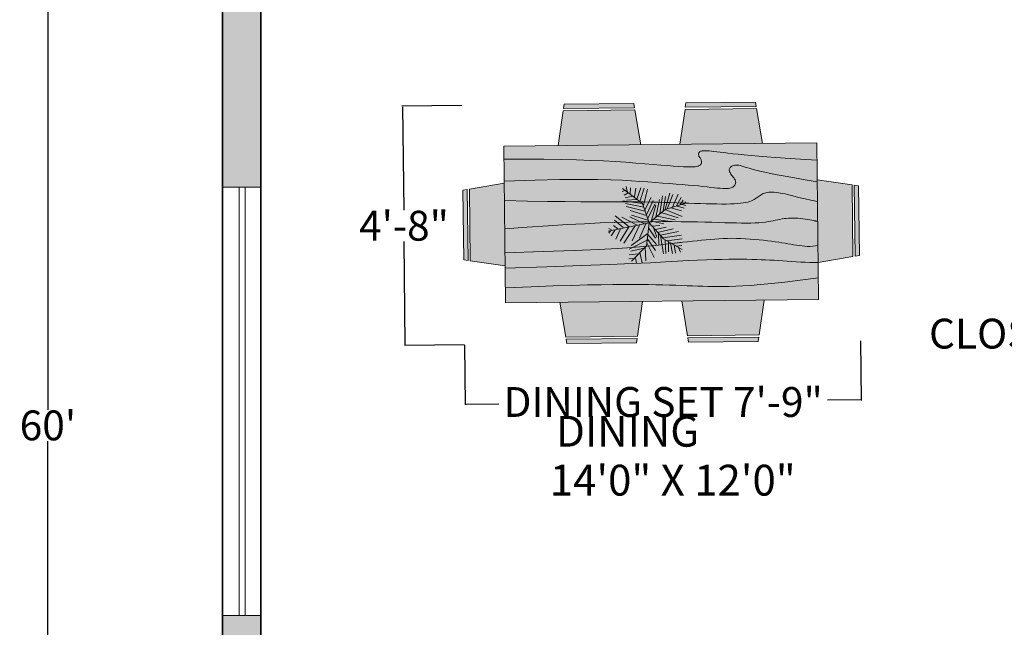
# Model space of a CAD drawing. Units: inches. Extents: x 2167 to 2589, y 1680 to 2489.
# Tile 32 of 38: x 2167 to 2399, y 2000 to 2143. Entities that reach past the tile are written whole.
import ezdxf

# ---------------------------------------------------------------- set-up
doc = ezdxf.new("R2010")
doc.units = ezdxf.units.IN
doc.header["$MEASUREMENT"] = 0
doc.layers.get('0').update_dxf_attribs({"color": 250})
for name, color, linetype, lineweight in [('A-ANNO-DIMS', 2, 'Continuous', 18), ('A-AREA-IDEN', 7, 'Continuous', 18), ('A-FURN-PATT', 31, 'Continuous', 13), ('A-WALL-PATT', 250, 'Continuous', 13), ('C-PROP', 7, 'Continuous', 35), ('furniture', 34, 'Continuous', 18), ('L-PLNT', 106, 'Continuous', 13), ('walls', 7, 'Continuous', 35), ('windows', 141, 'Continuous', 18)]:
    doc.layers.add(name, color=color, linetype=linetype, lineweight=lineweight)
doc.styles.get("Standard").update_dxf_attribs({"font": 'arial.ttf'})
doc.dimstyles.get("Standard").update_dxf_attribs({"dimtxt": 7, "dimasz": 0.18, "dimexe": 0.18, "dimexo": 0.0625, "dimgap": 0.09, "dimtad": 0, "dimtih": 1, "dimtoh": 1, "dimdec": 1, "dimzin": 0, "dimdsep": 46, "dimlunit": 3, "dimtxsty": 'Standard', "dimcen": 0.09, "dimadec": 0, "dimazin": 0, "dimtfac": 1, "dimtdec": 1, "dimtofl": 0, "dimtmove": 0, "dimatfit": 3, "dimfxl": 1, "dimtolj": 1, "dimtzin": 0, "dimarcsym": 0})

# ---------------------------------------------------------------- blocks, each defined once
blk = doc.blocks.new('Dining Set - 36 x 72 in.')
for p, q in [((-22, 27.5), (-22.1562, 26.50042)), ((-22, 27.5), (-6, 27.5)), ((-5.8437, 26.49966), (-6, 27.5)), ((6, 27.5), (5.8438, 26.50042)), ((6, 27.5), (22, 27.5)), ((22.1563, 26.49966), (22, 27.5)), ((-22.2343, 26.00059), (-23.4847, 17.99762)), ((-22.2304, 26), (-5.7608, 26)), ((-5.8416, 26.5), (-22.1534, 26.5)), ((-4.5152, 17.99762), (-5.7655, 25.99926)), ((5.7657, 26.00059), (4.5153, 17.99762)), ((5.7696, 26), (22.2392, 26)), ((22.1584, 26.5), (5.8466, 26.5)), ((23.4848, 17.99762), (22.2345, 25.99926)), ((36, 18), (-36, 18)), ((-36, 18), (-36, -18)), ((36, -18), (36, 18)), ((-44.0006, 8.23428), (-35.9976, 9.48474)), ((44.0006, 8.23428), (35.9976, 9.48474)), ((-45.5, 8), (-44.5004, 8.15617)), ((-45.5, 8), (-45.5, -8)), ((-44.5, -8.15843), (-44.5, 8.15338)), ((-44, 8.23041), (-44, -8.23915)), ((44, 8.23041), (44, -8.23915)), ((44.5, -8.15843), (44.5, 8.15338)), ((45.5, 8), (44.5005, 8.15617)), ((45.5, 8), (45.5, -8)), ((-44.4997, -8.15631), (-45.5, -8)), ((-35.9976, -9.48476), (-43.9993, -8.2345)), ((35.9976, -9.48476), (43.9993, -8.2345)), ((44.4997, -8.15631), (45.5, -8)), ((-36, -18), (36, -18)), ((-22.2343, -26.0006), (-23.4847, -17.99762)), ((-4.5152, -17.99762), (-5.7655, -25.99928)), ((5.7657, -26.0006), (4.5153, -17.99762)), ((23.4848, -17.99762), (22.2345, -25.99928)), ((-22.2304, -26), (-5.7608, -26)), ((-22, -27.5), (-22.1562, -26.50044)), ((-5.8416, -26.5), (-22.1534, -26.5)), ((-5.8437, -26.49967), (-6, -27.5)), ((5.7696, -26), (22.2392, -26)), ((6, -27.5), (5.8438, -26.50044)), ((22.1584, -26.5), (5.8466, -26.5)), ((22.1563, -26.49967), (22, -27.5)), ((-22, -27.5), (-6, -27.5)), ((6, -27.5), (22, -27.5))]:
    blk.add_line(p, q)
for points in [[(-36, 15), (-31.1772, 14.97754), (-26.8079, 14.91406), (-22.8538, 14.81543), (-19.276, 14.6875), (-16.0362, 14.53613), (-13.0957, 14.36718), (-10.4159, 14.18652), (-7.9583, 14), (-5.6904, 13.81315), (-3.6035, 13.63021), (-1.6954, 13.45508), (0.0365, 13.29166), (1.5945, 13.14388), (2.9811, 13.01562), (4.1988, 12.9108), (5.25, 12.83333), (6.1393, 12.78613), (6.8802, 12.76823), (7.4883, 12.77767), (7.9792, 12.8125), (8.3685, 12.87077), (8.6719, 12.95052), (8.9049, 13.0498), (9.0833, 13.16666), (9.2205, 13.29899), (9.3216, 13.44401), (9.3895, 13.59879), (9.4271, 13.76041), (9.4373, 13.92594), (9.4232, 14.09245), (9.3875, 14.257), (9.3333, 14.41666), (9.2638, 14.56917), (9.1836, 14.71484), (9.0975, 14.85465), (9.0104, 14.98958), (8.9272, 15.1206), (8.8529, 15.2487), (8.7922, 15.37483), (8.75, 15.5), (8.7305, 15.62467), (8.7344, 15.74739), (8.7617, 15.86621), (8.8125, 15.97916), (8.8867, 16.08431), (8.9844, 16.17968), (9.1055, 16.26334), (9.25, 16.33333), (9.4189, 16.38802), (9.6172, 16.42708), (9.8506, 16.45052), (10.125, 16.45833), (10.4463, 16.45052), (10.8203, 16.42708), (11.2529, 16.38802), (11.75, 16.33333), (12.3184, 16.26318), (12.9694, 16.17838), (13.7151, 16.07991), (14.5677, 15.96875), (15.5395, 15.84586), (16.6426, 15.71224), (17.8893, 15.56884), (19.2917, 15.41666), (20.859, 15.25667), (22.5879, 15.08984), (24.4721, 14.91715), (26.5052, 14.73958), (28.6809, 14.5581), (30.9929, 14.3737), (33.4347, 14.18733), (36, 14)], [(-36, 10), (-28.9766, 10.14274), (-23.1725, 10.20442), (-18.4241, 10.19775), (-14.5677, 10.13541), (-11.4399, 10.03011), (-8.877, 9.89453), (-6.7154, 9.74137), (-4.7917, 9.58333), (-2.9698, 9.43082), (-1.2246, 9.28515), (0.4415, 9.14534), (2.026, 9.01041), (3.5266, 8.87939), (4.9408, 8.7513), (6.266, 8.62516), (7.5, 8.5), (8.6411, 8.37549), (9.6914, 8.2539), (10.6538, 8.13818), (11.5312, 8.03125), (12.3267, 7.93603), (13.043, 7.85547), (13.6831, 7.79248), (14.25, 7.75), (14.7471, 7.7303), (15.1797, 7.73307), (15.5537, 7.75732), (15.875, 7.80208), (16.1494, 7.86637), (16.3828, 7.94922), (16.5811, 8.04964), (16.75, 8.16666), (16.8944, 8.29915), (17.0143, 8.44531), (17.1089, 8.60319), (17.1771, 8.77083), (17.218, 8.94629), (17.2305, 9.1276), (17.2137, 9.31282), (17.1667, 9.5), (17.0895, 9.6875), (16.987, 9.875), (16.8649, 10.0625), (16.7292, 10.25), (16.5856, 10.4375), (16.4401, 10.625), (16.2985, 10.8125), (16.1667, 11), (16.05, 11.18733), (15.9518, 11.3737), (15.8752, 11.5581), (15.8229, 11.73958), (15.798, 11.91715), (15.8034, 12.08984), (15.842, 12.25667), (15.9167, 12.41666), (16.0295, 12.56836), (16.1784, 12.70833), (16.3605, 12.83268), (16.5729, 12.9375), (16.8127, 13.01888), (17.0768, 13.07291), (17.3625, 13.0957), (17.6667, 13.08333), (17.9894, 13.03312), (18.3418, 12.94726), (18.7382, 12.82918), (19.1927, 12.68229), (19.7195, 12.51001), (20.3327, 12.31575), (21.0465, 12.10294), (21.875, 11.875), (22.8357, 11.63354), (23.959, 11.37304), (25.2786, 11.08618), (26.8282, 10.76562), (28.6414, 10.40405), (30.752, 9.99414), (33.1936, 9.52856), (36, 9)], [(-36, 5.5), (-30.7157, 5.3348), (-26.069, 5.20963), (-21.9946, 5.11767), (-18.4271, 5.05208), (-15.3009, 5.00602), (-12.5508, 4.97265), (-10.1112, 4.94515), (-7.9167, 4.91666), (-5.909, 4.88167), (-4.0586, 4.83984), (-2.3429, 4.79215), (-0.7396, 4.73958), (0.7739, 4.6831), (2.22, 4.6237), (3.6213, 4.56233), (5, 4.5), (6.373, 4.43782), (7.7344, 4.3776), (9.0723, 4.32129), (10.375, 4.27083), (11.6309, 4.22819), (12.8281, 4.19531), (13.9551, 4.17415), (15, 4.16666), (15.954, 4.17448), (16.819, 4.19791), (17.6001, 4.23698), (18.3021, 4.29166), (18.9299, 4.36198), (19.4883, 4.44791), (19.9823, 4.54948), (20.4167, 4.66666), (20.7969, 4.79899), (21.1302, 4.94401), (21.4245, 5.09879), (21.6875, 5.26041), (21.9271, 5.42594), (22.1511, 5.59245), (22.3672, 5.757), (22.5834, 5.91666), (22.8065, 6.06868), (23.0404, 6.21093), (23.2879, 6.34147), (23.5521, 6.45833), (23.8358, 6.55957), (24.142, 6.64323), (24.4735, 6.70735), (24.8334, 6.75), (25.2235, 6.76969), (25.642, 6.76692), (26.0858, 6.74267), (26.5521, 6.69791), (27.0379, 6.63362), (27.5404, 6.55078), (28.0565, 6.45036), (28.5834, 6.33333), (29.1242, 6.19987), (29.7071, 6.04687), (30.3661, 5.87044), (31.1354, 5.66666), (32.0493, 5.43164), (33.142, 5.16146), (34.4475, 4.85221), (36, 4.5)], [(-36, -1), (-30.7915, -0.6591), (-26.0195, -0.38216), (-21.6519, -0.16284), (-17.6563, 0.00521), (-14.0005, 0.12833), (-10.6523, 0.21289), (-7.5796, 0.26522), (-4.75, 0.29166), (-2.134, 0.29793), (0.2878, 0.28711), (2.5317, 0.26163), (4.6146, 0.22396), (6.5529, 0.17651), (8.3633, 0.12174), (10.0623, 0.06209), (11.6667, 0), (13.1899, -0.06201), (14.6341, -0.1211), (15.9982, -0.17432), (17.2813, -0.21875), (18.4823, -0.25147), (19.6003, -0.26953), (20.6343, -0.27002), (21.5834, -0.25), (22.4481, -0.20768), (23.2357, -0.14584), (23.9549, -0.06836), (24.6146, 0.02083), (25.2235, 0.11784), (25.7904, 0.21875), (26.3241, 0.31966), (26.8334, 0.41666), (27.3265, 0.50618), (27.8099, 0.58593), (28.2894, 0.65397), (28.7709, 0.70833), (29.2601, 0.74707), (29.763, 0.76823), (30.2855, 0.76985), (30.8334, 0.75), (31.4088, 0.70784), (31.9994, 0.64713), (32.589, 0.57275), (33.1615, 0.48958), (33.7008, 0.4025), (34.1908, 0.3164), (34.6153, 0.23616), (34.9584, 0.16666), (35.2099, 0.11165), (35.3848, 0.07031), (35.504, 0.04069), (35.5886, 0.02083), (35.6594, 0.00879), (35.7377, 0.0026), (35.8442, 0.00032), (36, 0)], [(-36, -6.5), (-27.1843, -6.31267), (-20.084, -6.1263), (-14.469, -5.9419), (-10.1094, -5.76042), (-6.7752, -5.58285), (-4.2363, -5.41016), (-2.2629, -5.24333), (-0.625, -5.08334), (0.8708, -4.93099), (2.2715, -4.78646), (3.5872, -4.64974), (4.8281, -4.52084), (6.0046, -4.39974), (7.127, -4.28646), (8.2053, -4.18099), (9.25, -4.08334), (10.2705, -3.99382), (11.2734, -3.91407), (12.2647, -3.84603), (13.25, -3.79167), (14.2354, -3.75293), (15.2266, -3.73177), (16.2295, -3.73015), (17.25, -3.75), (18.2912, -3.79248), (19.3451, -3.85547), (20.4009, -3.93604), (21.4479, -4.03125), (22.4754, -4.13819), (23.4727, -4.25391), (24.4289, -4.37549), (25.3334, -4.5), (26.1785, -4.62492), (26.9694, -4.74935), (27.7145, -4.87281), (28.4219, -4.99479), (29.1, -5.11483), (29.7572, -5.23242), (30.4016, -5.34709), (31.0417, -5.45834), (31.6837, -5.56437), (32.3262, -5.65821), (32.9658, -5.73153), (33.599, -5.77604), (34.2224, -5.78345), (34.8327, -5.74545), (35.4264, -5.65373), (36, -5.5)], [(-36, -10), (-26.4022, -9.81299), (-18.4675, -9.62891), (-11.9839, -9.45069), (-6.7396, -9.28125), (-2.5226, -9.12354), (0.8789, -8.98047), (3.6769, -8.85498), (6.0833, -8.75), (8.2767, -8.66765), (10.3021, -8.60677), (12.1712, -8.56543), (13.8958, -8.54167), (15.4876, -8.53353), (16.9583, -8.53907), (18.3197, -8.55632), (19.5834, -8.58334), (20.7616, -8.61841), (21.8685, -8.66081), (22.9188, -8.71004), (23.9271, -8.76563), (24.9081, -8.82707), (25.8763, -8.89388), (26.8465, -8.96558), (27.8334, -9.04167), (28.8474, -9.12118), (29.8828, -9.20117), (30.93, -9.27824), (31.9792, -9.34896), (33.0205, -9.40991), (34.0443, -9.45768), (35.0407, -9.48885), (36, -9.5)], [(-36, -14.5), (-30.0881, -14.33513), (-25.0332, -14.21224), (-20.7312, -14.12647), (-17.0781, -14.07292), (-13.97, -14.04671), (-11.3027, -14.04297), (-8.9724, -14.05681), (-6.875, -14.08334), (-4.9224, -14.11833), (-3.0905, -14.16016), (-1.3709, -14.20785), (0.2448, -14.26042), (1.7647, -14.3169), (3.1973, -14.3763), (4.5507, -14.43767), (5.8333, -14.5), (7.0554, -14.5621), (8.235, -14.62175), (9.3922, -14.67652), (10.5469, -14.72396), (11.7192, -14.76164), (12.929, -14.78711), (14.1965, -14.79794), (15.5417, -14.79167), (16.9933, -14.76424), (18.6152, -14.70508), (20.4804, -14.60197), (22.6615, -14.44271), (25.2312, -14.21509), (28.2624, -13.9069), (31.8277, -13.50594), (36, -13)]]:
    blk.add_lwpolyline(points)
blk = doc.blocks.new('dining area')
at = {"layer": 'furniture', "xscale": 0.6659924291999282, "yscale": 0.6659924291999282, "zscale": 0.6659924291999282, "rotation": 90}
blk.add_blockref('Dining Set - 36 x 72 in.', (-0.44, 20.51), dxfattribs=at)
blk = doc.blocks.new('*U8')
for p, q in [((-10.186, 53.64), (-13.084, 55.962)), ((0, 0), (-10.5, 57)), ((-9.099, 51.782), (-6.563, 55.962)), ((-7.288, 39.707), (-21.778, 46.673)), ((-8.737, 47.138), (-17.069, 52.711)), ((-7.65, 43.423), (-2.578, 49.46)), ((-5.839, 35.992), (4.667, 48.067)), ((-5.114, 27.632), (10.463, 46.673)), ((-48.585, 21.131), (-49.309, 29.026)), ((-43.513, 28.561), (-42.427, 15.558)), ((-35.544, 28.097), (-24.314, 3.947)), ((-3.665, 19.273), (-27.574, 35.527)), ((-5.114, 28.097), (-24.676, 40.636)), ((-2.941, 16.486), (8.652, 37.85)), ((16.259, 5.805), (23.142, 31.348)), ((22.055, 7.198), (27.489, 32.277)), ((27, 9), (48, 36)), ((27.127, 9.056), (31.112, 35.992)), ((31.836, 30.883), (32.561, 16.486)), ((35.096, 32.741), (37.27, 22.524)), ((38.719, 34.134), (41.979, 28.561)), ((43.791, 29.954), (51.036, 30.883)), ((44.153, 36.456), (45.239, 32.741)), ((-47.498, 19.737), (-55.83, 18.344)), ((-40.615, 13.7), (-55.105, 10.913)), ((-31.5, 4.5), (-52.5, 25.5)), ((-38.442, 26.239), (-34.819, 7.663)), ((-14.533, 2.09), (-30.834, 25.31)), ((-24.314, 23.917), (-2.941, 13.7)), ((-20.691, 13.7), (-1.129, 4.876)), ((-1.129, 6.734), (9.014, 26.704)), ((3.942, 1.625), (11.187, 24.381)), ((10.101, 3.483), (17.708, 26.239)), ((33.285, 16.486), (48.862, 10.913)), ((36.183, 19.737), (48.137, 17.88)), ((40.53, 25.775), (48.862, 24.846)), ((-33.37, 6.269), (-52.207, 5.34)), ((-28.299, 3.483), (-47.86, -5.805)), ((-21.416, 3.018), (-38.079, -8.128)), ((0, 0), (-31.5, 4.5)), ((-15.982, 2.09), (-30.11, -9.521)), ((0, 0), (-22.5, -19.5)), ((-6.563, 1.161), (-21.416, -8.128)), ((0, 0), (27, 9)), ((0, 0), (18, -22.5)), ((6.478, 1.625), (26.04, -8.592)), ((11.187, 3.483), (30.749, -5.805)), ((18.07, 5.805), (35.096, -3.483)), ((24.229, 7.663), (46.688, 1.625)), ((29.662, 12.307), (48.137, 6.269)), ((-15.257, -12.772), (-30.11, -12.772)), ((-6.563, -5.805), (-19.967, -9.985)), ((-13.446, -11.378), (-8.737, -32.741)), ((-9.461, -8.592), (-6.201, -23.453)), ((-4.752, -3.483), (-3.665, -14.629)), ((2.493, -3.019), (-1.491, -20.202)), ((1.769, -2.555), (24.229, -9.521)), ((5.029, -6.27), (2.131, -25.775)), ((9.014, -11.378), (3.58, -35.992)), ((7.565, -9.056), (32.198, -14.629)), ((-17.431, -15.094), (-42.789, -18.809)), ((-24.314, -21.596), (-42.427, -22.06)), ((-26.849, -26.24), (-40.253, -25.775)), ((-22.5, -19.5), (-37.5, -45)), ((-25.038, -23.918), (-22.865, -45.281)), ((-20.691, -18.345), (-17.793, -44.352)), ((-17.069, -15.094), (-12.721, -40.172)), ((14.085, -16.951), (6.478, -40.172)), ((18.07, -22.524), (8.289, -45.745)), ((12.274, -15.094), (36.907, -18.809)), ((16.259, -19.738), (36.183, -22.989)), ((18, -22.5), (27, -52.5)), ((18.433, -22.524), (40.53, -29.026)), ((19.157, -25.311), (38.719, -33.206)), ((-28.299, -29.026), (-42.789, -31.348)), ((-30.834, -34.135), (-42.427, -35.528)), ((-34.457, -39.708), (-40.978, -42.494)), ((-32.646, -36.921), (-31.921, -44.352)), ((-29.023, -30.884), (-27.936, -43.887)), ((20.244, -30.419), (15.897, -44.816)), ((22.78, -37.85), (19.519, -48.532)), ((21.331, -32.741), (39.081, -40.636)), ((22.78, -38.314), (34.372, -44.816)), ((24.591, -45.745), (23.142, -50.854)), ((24.591, -43.423), (30.749, -47.603)), ((26.764, -49.925), (28.213, -50.854))]:
    blk.add_line(p, q)
blk = doc.blocks.new('*D24')
at = {"layer": 'A-ANNO-DIMS', "color": 0, "lineweight": -2, "transparency": 16777216}
for p, q in [((2174.43, 2407.69), (2173.89, 2407.69)), ((2174.07, 2407.51), (2174.07, 2051.36)), ((2174.07, 1687.87), (2174.07, 2044.03)), ((2174.43, 1687.69), (2173.89, 1687.69))]:
    blk.add_line(p, q, dxfattribs=at)
at = {"layer": 'A-ANNO-DIMS', "color": 0, "transparency": 16777216}
for points in [[(2174.04, 2407.51), (2174.1, 2407.51), (2174.07, 2407.69)], [(2174.04, 1687.87), (2174.1, 1687.87), (2174.07, 1687.69)]]:
    blk.add_solid(points, dxfattribs=at)
at = {"layer": 'Defpoints', "color": 0, "transparency": 16777216}
for p in [(2174.49, 2407.69), (2174.07, 1687.69), (2174.49, 1687.69)]:
    blk.add_point(p, dxfattribs=at)
at = {"layer": 'A-ANNO-DIMS', "color": 0, "transparency": 16777216, "insert": (2174.07, 2047.69), "char_height": 7, "attachment_point": 5}
blk.add_mtext("\\A1;60'", dxfattribs=at)
blk = doc.blocks.new('*D35')
at = {"layer": 'A-ANNO-DIMS', "color": 0, "lineweight": -2, "transparency": 16777216}
for p, q in [((2422.18, 2109.24), (2410.06, 2109.24)), ((2410.24, 2109.06), (2410.24, 2072.94)), ((2410.24, 2029.39), (2410.24, 2065.51)), ((2422.18, 2029.21), (2410.06, 2029.21))]:
    blk.add_line(p, q, dxfattribs=at)
at = {"layer": 'A-ANNO-DIMS', "color": 0, "transparency": 16777216}
for points in [[(2410.21, 2109.06), (2410.27, 2109.06), (2410.24, 2109.24)], [(2410.21, 2029.39), (2410.27, 2029.39), (2410.24, 2029.21)]]:
    blk.add_solid(points, dxfattribs=at)
at = {"layer": 'Defpoints', "color": 0, "transparency": 16777216}
for p in [(2422.24, 2109.24), (2410.24, 2029.21), (2422.24, 2029.21)]:
    blk.add_point(p, dxfattribs=at)
at = {"layer": 'A-ANNO-DIMS', "color": 0, "transparency": 16777216, "insert": (2410.24, 2069.22), "char_height": 7, "attachment_point": 5}
blk.add_mtext('\\A1;CLOSET 6\'-8"', dxfattribs=at)
blk = doc.blocks.new('*D51')
at = {"layer": 'A-ANNO-DIMS', "color": 0, "lineweight": -2, "transparency": 16777216}
for p, q in [((2271.9, 2066.54), (2272.06, 2052.48)), ((2364.8, 2067.56), (2364.96, 2053.51)), ((2272.24, 2052.67), (2279.95, 2052.75)), ((2364.77, 2053.69), (2357.06, 2053.6))]:
    blk.add_line(p, q, dxfattribs=at)
at = {"layer": 'A-ANNO-DIMS', "color": 0, "transparency": 16777216}
for points in [[(2272.24, 2052.7), (2272.24, 2052.64), (2272.06, 2052.66)], [(2364.77, 2053.72), (2364.77, 2053.66), (2364.95, 2053.69)]]:
    blk.add_solid(points, dxfattribs=at)
at = {"layer": 'Defpoints', "color": 0, "transparency": 16777216}
for p in [(2271.9, 2066.6), (2364.8, 2067.63), (2364.95, 2053.69)]:
    blk.add_point(p, dxfattribs=at)
at = {"layer": 'A-ANNO-DIMS', "color": 0, "transparency": 16777216, "insert": (2318.5, 2053.18), "char_height": 7, "attachment_point": 5}
blk.add_mtext('\\A1;DINING SET 7\'-9"', dxfattribs=at)
blk = doc.blocks.new('*D52')
at = {"layer": 'A-ANNO-DIMS', "color": 0, "lineweight": -2, "transparency": 16777216}
for p, q in [((2271.22, 2122.74), (2257.17, 2122.59)), ((2257.35, 2122.41), (2257.62, 2098.18)), ((2257.97, 2066.63), (2257.7, 2090.85)), ((2271.84, 2066.6), (2257.79, 2066.44))]:
    blk.add_line(p, q, dxfattribs=at)
at = {"layer": 'A-ANNO-DIMS', "color": 0, "transparency": 16777216}
for points in [[(2257.38, 2122.41), (2257.32, 2122.41), (2257.35, 2122.59)], [(2258, 2066.63), (2257.94, 2066.62), (2257.97, 2066.45)]]:
    blk.add_solid(points, dxfattribs=at)
at = {"layer": 'Defpoints', "color": 0, "transparency": 16777216}
for p in [(2271.28, 2122.75), (2271.9, 2066.6), (2257.97, 2066.45)]:
    blk.add_point(p, dxfattribs=at)
at = {"layer": 'A-ANNO-DIMS', "color": 0, "transparency": 16777216, "insert": (2257.66, 2094.52), "char_height": 7, "attachment_point": 5}
blk.add_mtext('\\A1;4\'-8"', dxfattribs=at)

msp = doc.modelspace()

# ---------------------------------------------------------------- hatches: boundary and pattern name
at = {"layer": 'A-FURN-PATT'}
h = msp.add_hatch(color=256, dxfattribs=at)
h.dxf.hatch_style = 1
h.paths.add_polyline_path([(2311.86, 2121.66), (2295.05, 2121.48), (2293.86, 2113.3), (2313.23, 2113.51)])
h.paths.add_polyline_path([(2311.6, 2123.19), (2295.27, 2123.01), (2295.12, 2121.99), (2311.78, 2122.17)])
h.paths.add_polyline_path([(2340.44, 2121.98), (2323.63, 2121.79), (2322.45, 2113.61), (2341.81, 2113.83)])
h.paths.add_polyline_path([(2340.19, 2123.51), (2323.85, 2123.33), (2323.71, 2122.3), (2340.36, 2122.49)])
h.paths.add_polyline_path([(2281.18, 2104.46), (2273.03, 2103.1), (2273.22, 2086.28), (2281.4, 2085.1)])
h.paths.add_polyline_path([(2272.52, 2103.01), (2271.5, 2102.84), (2271.68, 2086.51), (2272.71, 2086.36)])
h.paths.add_polyline_path([(2313.63, 2076.76), (2294.27, 2076.55), (2295.64, 2068.39), (2312.45, 2068.58)])
h.paths.add_polyline_path([(2312.37, 2068.07), (2295.72, 2067.88), (2295.89, 2066.86), (2312.23, 2067.05)])
h.paths.add_polyline_path([(2340.96, 2068.38), (2324.31, 2068.2), (2324.48, 2067.18), (2340.81, 2067.36)])
h.paths.add_polyline_path([(2342.22, 2077.08), (2322.85, 2076.86), (2324.22, 2068.71), (2341.03, 2068.9)])
h.paths.add_polyline_path([(2364.4, 2103.87), (2363.38, 2104.01), (2363.56, 2087.36), (2364.58, 2087.53)])
h.paths.add_polyline_path([(2362.86, 2104.09), (2354.68, 2105.27), (2354.9, 2085.91), (2363.05, 2087.28)])
h = msp.add_hatch(color=256, dxfattribs=at)
h.dxf.hatch_style = 1
h.paths.add_polyline_path([(2281.45, 2079.98), (2287.49, 2080.21), (2292.65, 2080.39), (2297.04, 2080.53), (2300.77, 2080.63), (2303.94, 2080.69), (2306.66, 2080.72), (2309.04, 2080.73), (2311.18, 2080.73), (2313.17, 2080.72), (2315.05, 2080.7), (2316.8, 2080.67), (2318.45, 2080.63), (2320, 2080.59), (2321.47, 2080.55), (2322.85, 2080.5), (2324.16, 2080.45), (2325.41, 2080.4), (2326.61, 2080.35), (2327.79, 2080.31), (2328.97, 2080.27), (2330.17, 2080.25), (2331.41, 2080.24), (2332.7, 2080.24), (2334.07, 2080.26), (2335.55, 2080.31), (2337.21, 2080.38), (2339.11, 2080.51), (2341.34, 2080.7), (2343.96, 2080.96), (2347.05, 2081.31), (2350.68, 2081.76), (2354.94, 2082.32), (2354.85, 2089.98), (2354.27, 2089.81), (2353.66, 2089.71), (2353.04, 2089.67), (2352.4, 2089.67), (2351.76, 2089.71), (2351.1, 2089.77), (2350.45, 2089.86), (2349.79, 2089.96), (2349.14, 2090.07), (2348.48, 2090.18), (2347.8, 2090.29), (2347.11, 2090.41), (2346.39, 2090.52), (2345.63, 2090.64), (2344.82, 2090.76), (2343.95, 2090.88), (2343.03, 2091), (2342.05, 2091.11), (2341.03, 2091.22), (2339.98, 2091.31), (2338.91, 2091.4), (2337.83, 2091.47), (2336.76, 2091.52), (2335.69, 2091.55), (2334.65, 2091.56), (2333.63, 2091.55), (2332.61, 2091.52), (2331.61, 2091.46), (2330.6, 2091.4), (2329.59, 2091.32), (2328.57, 2091.22), (2327.53, 2091.12), (2326.46, 2091.01), (2325.36, 2090.89), (2324.22, 2090.76), (2323.02, 2090.63), (2321.75, 2090.48), (2320.41, 2090.33), (2318.98, 2090.16), (2317.4, 2089.98), (2317.7, 2088.47), (2317.63, 2088.51), (2317.68, 2088.58), (2317.4, 2089.98), (2315.79, 2089.81), (2313.78, 2089.62), (2311.19, 2089.41), (2307.79, 2089.19), (2303.34, 2088.96), (2297.61, 2088.71), (2290.36, 2088.43), (2281.36, 2088.14)])
h.paths.add_polyline_path([(2281.49, 2076.4), (2354.99, 2077.22), (2354.94, 2082.32), (2350.68, 2081.76), (2347.05, 2081.31), (2343.96, 2080.96), (2341.34, 2080.7), (2339.11, 2080.51), (2337.21, 2080.38), (2335.55, 2080.31), (2334.07, 2080.26), (2332.7, 2080.24), (2331.41, 2080.24), (2330.17, 2080.25), (2328.97, 2080.27), (2327.79, 2080.31), (2326.61, 2080.35), (2325.41, 2080.4), (2324.16, 2080.45), (2322.85, 2080.5), (2321.47, 2080.55), (2320, 2080.59), (2318.45, 2080.63), (2316.8, 2080.67), (2315.05, 2080.7), (2313.17, 2080.72), (2311.18, 2080.73), (2309.04, 2080.73), (2306.66, 2080.72), (2303.94, 2080.69), (2300.77, 2080.63), (2297.04, 2080.53), (2292.65, 2080.39), (2287.49, 2080.21), (2281.45, 2079.98)])
h.paths.add_polyline_path([(2321.25, 2094.18), (2323.53, 2093.89), (2326.51, 2091.01), (2327.53, 2091.12), (2328.57, 2091.22), (2329.59, 2091.32), (2330.6, 2091.4), (2331.61, 2091.46), (2332.61, 2091.52), (2333.63, 2091.55), (2334.65, 2091.56), (2335.69, 2091.55), (2336.76, 2091.52), (2337.83, 2091.47), (2338.91, 2091.4), (2339.98, 2091.31), (2341.03, 2091.22), (2342.05, 2091.11), (2343.03, 2091), (2343.95, 2090.88), (2344.82, 2090.76), (2345.63, 2090.64), (2346.39, 2090.52), (2347.11, 2090.41), (2347.8, 2090.29), (2348.48, 2090.18), (2349.14, 2090.07), (2349.79, 2089.96), (2350.45, 2089.86), (2351.1, 2089.77), (2351.76, 2089.71), (2352.4, 2089.67), (2353.04, 2089.67), (2353.66, 2089.71), (2354.27, 2089.81), (2354.85, 2089.98), (2354.79, 2095.59), (2354.49, 2095.59), (2354.36, 2095.61), (2354.16, 2095.66), (2353.98, 2095.7), (2353.73, 2095.75), (2353.37, 2095.82), (2352.94, 2095.89), (2352.44, 2095.98), (2351.89, 2096.06), (2351.3, 2096.14), (2350.7, 2096.21), (2350.1, 2096.26), (2349.51, 2096.3), (2348.95, 2096.31), (2348.41, 2096.31), (2347.9, 2096.28), (2347.4, 2096.23), (2346.91, 2096.17), (2346.42, 2096.1), (2345.93, 2096.01), (2345.43, 2095.91), (2344.91, 2095.81), (2344.37, 2095.7), (2343.79, 2095.59), (2343.17, 2095.49), (2342.5, 2095.39), (2341.76, 2095.3), (2340.96, 2095.23), (2340.08, 2095.17), (2339.11, 2095.14), (2338.05, 2095.13), (2336.91, 2095.14), (2335.68, 2095.16), (2334.37, 2095.19), (2332.98, 2095.23), (2331.51, 2095.27), (2329.95, 2095.32), (2328.31, 2095.36), (2326.58, 2095.4), (2324.73, 2095.44), (2323.1, 2095.46)])
h.paths.add_polyline_path([(2281.36, 2088.14), (2290.36, 2088.43), (2297.61, 2088.71), (2303.34, 2088.96), (2307.79, 2089.19), (2307.79, 2089.19), (2310.36, 2092.61), (2310.36, 2092.64), (2312.44, 2093.37), (2308.71, 2095.33), (2307.16, 2095.28), (2303.75, 2095.16), (2300.02, 2094.99), (2295.94, 2094.78), (2291.48, 2094.5), (2286.61, 2094.17), (2281.3, 2093.76)])
h.paths.add_polyline_path([(2281.3, 2093.76), (2286.61, 2094.17), (2291.48, 2094.5), (2295.94, 2094.78), (2300.02, 2094.99), (2303.75, 2095.16), (2307.16, 2095.28), (2310.3, 2095.37), (2313.19, 2095.43), (2315.86, 2095.47), (2312.28, 2099.79), (2312.27, 2099.76), (2310.98, 2100.11), (2309.9, 2100.12), (2307.66, 2100.12), (2305.17, 2100.12), (2302.36, 2100.12), (2299.17, 2100.14), (2295.53, 2100.16), (2291.37, 2100.21), (2286.62, 2100.29), (2281.23, 2100.39)])
h.paths.add_polyline_path([(2281.23, 2100.39), (2286.62, 2100.29), (2291.37, 2100.21), (2295.53, 2100.16), (2299.17, 2100.14), (2302.36, 2100.12), (2305.17, 2100.12), (2307.66, 2100.12), (2309.9, 2100.12), (2310.98, 2100.11), (2312.27, 2099.76), (2312.28, 2099.79), (2315.86, 2095.47), (2318.33, 2095.48), (2320.62, 2095.48), (2322.75, 2095.47), (2324.73, 2095.44), (2326.58, 2095.4), (2328.31, 2095.36), (2329.95, 2095.32), (2331.51, 2095.27), (2332.98, 2095.23), (2334.37, 2095.19), (2335.68, 2095.16), (2336.91, 2095.14), (2338.05, 2095.13), (2339.11, 2095.14), (2340.08, 2095.17), (2340.96, 2095.23), (2341.76, 2095.3), (2342.5, 2095.39), (2343.17, 2095.49), (2343.79, 2095.59), (2344.37, 2095.7), (2344.91, 2095.81), (2345.43, 2095.91), (2345.93, 2096.01), (2346.42, 2096.1), (2346.91, 2096.17), (2347.4, 2096.23), (2347.9, 2096.28), (2348.41, 2096.31), (2348.95, 2096.31), (2349.51, 2096.3), (2350.1, 2096.26), (2350.7, 2096.21), (2351.3, 2096.14), (2351.89, 2096.06), (2352.44, 2095.98), (2352.94, 2095.89), (2353.37, 2095.82), (2353.73, 2095.75), (2353.98, 2095.7), (2354.16, 2095.66), (2354.28, 2095.63), (2354.37, 2095.61), (2354.44, 2095.6), (2354.52, 2095.59), (2354.63, 2095.59), (2354.79, 2095.59), (2354.63, 2109.88), (2352.01, 2110.05), (2349.52, 2110.21), (2347.15, 2110.37), (2344.93, 2110.53), (2342.85, 2110.69), (2340.93, 2110.85), (2339.16, 2111), (2337.56, 2111.14), (2336.13, 2111.28), (2334.85, 2111.41), (2333.72, 2111.54), (2332.73, 2111.65), (2331.86, 2111.76), (2331.1, 2111.85), (2330.43, 2111.93), (2329.85, 2111.99), (2329.34, 2112.04), (2328.9, 2112.08), (2328.52, 2112.1), (2328.19, 2112.1), (2327.91, 2112.09), (2327.67, 2112.06), (2327.47, 2112.02), (2327.3, 2111.96), (2327.15, 2111.89), (2327.03, 2111.8), (2326.93, 2111.71), (2326.86, 2111.6), (2326.81, 2111.48), (2326.78, 2111.36), (2326.78, 2111.23), (2326.8, 2111.11), (2326.84, 2110.98), (2326.91, 2110.85), (2326.98, 2110.72), (2327.07, 2110.59), (2327.22, 2110.36), (2327.38, 2110.08), (2327.49, 2109.76), (2327.53, 2109.42), (2327.47, 2109.17), (2327.4, 2109.02), (2327.3, 2108.87), (2327.16, 2108.73), (2326.98, 2108.61), (2326.75, 2108.5), (2326.44, 2108.42), (2326.04, 2108.36), (2325.54, 2108.31), (2324.92, 2108.3), (2324.16, 2108.31), (2323.25, 2108.35), (2322.18, 2108.41), (2320.94, 2108.51), (2319.52, 2108.62), (2317.93, 2108.75), (2316.16, 2108.9), (2314.21, 2109.06), (2312.08, 2109.22), (2309.76, 2109.39), (2307.25, 2109.55), (2304.51, 2109.7), (2301.51, 2109.84), (2298.2, 2109.96), (2294.54, 2110.05), (2290.51, 2110.11), (2286.04, 2110.12), (2281.12, 2110.09)])
h.paths.add_polyline_path([(2311.08, 2105.05), (2313.04, 2104.91), (2314.9, 2104.78), (2316.69, 2104.65), (2318.39, 2104.53), (2320.01, 2104.41), (2321.49, 2104.29), (2321.49, 2104.29), (2322.99, 2104.18), (2324.34, 2104.06), (2324.48, 2104.05), (2324.01, 2103.84), (2321.97, 2100.24), (2321.49, 2104.29), (2320.01, 2104.41), (2318.39, 2104.53), (2316.69, 2104.65), (2314.9, 2104.78), (2313.04, 2104.91), (2311.67, 2105.01), (2311.17, 2103.27), (2310.6, 2105.08)], flags=16)
h.paths.add_polyline_path([(2281.12, 2110.09), (2286.04, 2110.12), (2290.51, 2110.11), (2294.54, 2110.05), (2298.2, 2109.96), (2301.51, 2109.84), (2304.51, 2109.7), (2307.25, 2109.55), (2309.76, 2109.39), (2312.08, 2109.22), (2314.21, 2109.06), (2316.16, 2108.9), (2317.93, 2108.75), (2319.52, 2108.62), (2320.94, 2108.51), (2322.18, 2108.41), (2323.25, 2108.35), (2324.16, 2108.31), (2324.92, 2108.3), (2325.54, 2108.31), (2326.04, 2108.36), (2326.44, 2108.42), (2326.75, 2108.5), (2326.98, 2108.61), (2327.16, 2108.73), (2327.3, 2108.87), (2327.4, 2109.02), (2327.47, 2109.17), (2327.51, 2109.34), (2327.52, 2109.51), (2327.5, 2109.68), (2327.46, 2109.85), (2327.41, 2110.01), (2327.33, 2110.16), (2327.25, 2110.31), (2327.16, 2110.45), (2327, 2110.7), (2326.86, 2110.93), (2326.78, 2111.17), (2326.78, 2111.42), (2326.88, 2111.66), (2327.08, 2111.86), (2327.3, 2111.96), (2327.47, 2112.02), (2327.67, 2112.06), (2327.91, 2112.09), (2328.19, 2112.1), (2328.52, 2112.1), (2328.9, 2112.08), (2329.34, 2112.04), (2329.85, 2111.99), (2330.43, 2111.93), (2331.1, 2111.85), (2331.86, 2111.76), (2332.73, 2111.65), (2333.72, 2111.54), (2334.85, 2111.41), (2336.13, 2111.28), (2337.56, 2111.14), (2339.16, 2111), (2340.93, 2110.85), (2342.85, 2110.69), (2344.93, 2110.53), (2347.15, 2110.37), (2349.52, 2110.21), (2352.01, 2110.05), (2354.63, 2109.88), (2354.59, 2113.97), (2281.09, 2113.15)])
h.paths.add_polyline_path([(2307.79, 2089.19), (2311.19, 2089.41), (2313.78, 2089.62), (2315.79, 2089.81), (2317.46, 2089.99), (2318.98, 2090.16), (2320.41, 2090.33), (2321.75, 2090.48), (2323.02, 2090.63), (2324.22, 2090.76), (2325.36, 2090.89), (2326.51, 2091.02), (2323.53, 2093.89), (2321.25, 2094.18), (2323.1, 2095.46), (2322.75, 2095.47), (2320.62, 2095.48), (2318.33, 2095.48), (2315.86, 2095.47), (2313.19, 2095.43), (2310.3, 2095.37), (2308.71, 2095.33), (2312.44, 2093.37), (2310.39, 2092.65)])
h.paths.add_polyline_path([(2321.97, 2100.24), (2324.01, 2103.84), (2324.48, 2104.05), (2324.34, 2104.06), (2322.99, 2104.18), (2321.49, 2104.29)], flags=0)
h.paths.add_polyline_path([(2311.17, 2103.27), (2311.67, 2105.01), (2311.08, 2105.05), (2310.6, 2105.08)], flags=0)
h = msp.add_hatch(color=256, dxfattribs=at)
h.dxf.hatch_style = 1
h.paths.add_polyline_path([(2281.23, 2100.39), (2286.62, 2100.29), (2291.37, 2100.21), (2295.53, 2100.16), (2299.17, 2100.14), (2302.36, 2100.12), (2305.17, 2100.12), (2307.66, 2100.12), (2309.9, 2100.12), (2311.95, 2100.1), (2313.84, 2100.08), (2315.59, 2100.05), (2317.23, 2100.02), (2318.78, 2099.98), (2320.25, 2099.93), (2321.69, 2099.88), (2323.09, 2099.84), (2324.5, 2099.79), (2325.89, 2099.74), (2327.25, 2099.7), (2328.58, 2099.66), (2329.87, 2099.63), (2331.09, 2099.61), (2332.24, 2099.6), (2333.31, 2099.61), (2334.28, 2099.63), (2335.16, 2099.66), (2335.96, 2099.71), (2336.68, 2099.77), (2337.32, 2099.85), (2337.88, 2099.95), (2338.39, 2100.06), (2338.83, 2100.18), (2339.22, 2100.32), (2339.56, 2100.47), (2339.85, 2100.63), (2340.12, 2100.8), (2340.36, 2100.97), (2340.59, 2101.14), (2340.81, 2101.32), (2341.03, 2101.48), (2341.25, 2101.64), (2341.49, 2101.79), (2341.74, 2101.92), (2342.01, 2102.04), (2342.3, 2102.15), (2342.61, 2102.24), (2342.95, 2102.31), (2343.32, 2102.36), (2343.71, 2102.38), (2344.14, 2102.38), (2344.59, 2102.36), (2345.07, 2102.32), (2345.57, 2102.26), (2346.08, 2102.18), (2346.61, 2102.09), (2347.15, 2101.97), (2347.7, 2101.84), (2348.3, 2101.69), (2348.97, 2101.52), (2349.76, 2101.32), (2350.7, 2101.09), (2351.81, 2100.83), (2353.15, 2100.53), (2354.74, 2100.19), (2354.69, 2104.78), (2351.82, 2105.29), (2349.32, 2105.74), (2347.16, 2106.13), (2345.31, 2106.48), (2343.72, 2106.79), (2342.37, 2107.07), (2341.22, 2107.32), (2340.24, 2107.56), (2339.39, 2107.78), (2338.66, 2107.99), (2338.03, 2108.18), (2337.49, 2108.35), (2337.02, 2108.49), (2336.62, 2108.61), (2336.26, 2108.69), (2335.93, 2108.74), (2335.62, 2108.75), (2335.33, 2108.72), (2335.06, 2108.67), (2334.81, 2108.58), (2334.6, 2108.47), (2334.41, 2108.34), (2334.26, 2108.2), (2334.15, 2108.04), (2334.07, 2107.88), (2334.04, 2107.71), (2334.03, 2107.53), (2334.06, 2107.35), (2334.12, 2107.16), (2334.2, 2106.98), (2334.3, 2106.79), (2334.42, 2106.6), (2334.56, 2106.41), (2334.7, 2106.22), (2334.85, 2106.03), (2335, 2105.84), (2335.14, 2105.65), (2335.27, 2105.46), (2335.38, 2105.27), (2335.46, 2105.08), (2335.51, 2104.89), (2335.53, 2104.7), (2335.52, 2104.51), (2335.48, 2104.33), (2335.41, 2104.16), (2335.31, 2104), (2335.19, 2103.85), (2335.05, 2103.71), (2334.88, 2103.59), (2334.67, 2103.49), (2334.44, 2103.4), (2334.16, 2103.33), (2333.83, 2103.28), (2333.45, 2103.25), (2333.01, 2103.24), (2332.5, 2103.26), (2331.92, 2103.3), (2331.27, 2103.35), (2330.53, 2103.43), (2329.72, 2103.51), (2328.82, 2103.61), (2327.84, 2103.72), (2326.77, 2103.83), (2325.6, 2103.95), (2324.34, 2104.06), (2322.99, 2104.18), (2321.54, 2104.29), (2320.01, 2104.41), (2318.39, 2104.53), (2316.69, 2104.65), (2314.9, 2104.78), (2313.04, 2104.91), (2311.08, 2105.05), (2308.87, 2105.19), (2306.25, 2105.3), (2303.05, 2105.37), (2299.12, 2105.39), (2294.27, 2105.34), (2288.35, 2105.21), (2281.18, 2104.99)])
at = {"layer": 'A-WALL-PATT'}
h = msp.add_hatch(color=256, dxfattribs=at)
h.dxf.hatch_style = 1
h.paths.add_polyline_path([(2575.05, 2029.69), (2422.05, 2029.69), (2422.05, 2161.69), (2427.02, 2161.69), (2427.02, 2161.94), (2427.02, 2166.19), (2417.55, 2166.19), (2417.55, 2025.19), (2575.05, 2025.19)])
h.paths.add_polyline_path([(2575.05, 2166.19), (2503.01, 2166.19), (2503.01, 2161.69), (2575.05, 2161.69)], flags=17)
h.paths.add_polyline_path([(2575.05, 2161.69), (2566.05, 2161.69), (2566.05, 2029.69), (2575.05, 2029.69)], flags=17)
h.paths.add_polyline_path([(2575.05, 2025.19), (2566.05, 2025.19), (2566.05, 1869.19), (2575.05, 1869.19)])
h.paths.add_polyline_path([(2575.05, 1869.19), (2566.05, 1869.19), (2447.7, 1869.19, -0.014764), (2447.74, 1867.92), (2447.74, 1864.69), (2575.05, 1864.69)])
h.paths.add_polyline_path([(2530.05, 1864.69), (2525.55, 1864.69), (2525.55, 1816.69), (2452.05, 1816.69), (2452.05, 1812.19), (2530.05, 1812.19)])
h.paths.add_polyline_path([(2455.04, 1830.65), (2452.05, 1830.65), (2452.05, 1816.69), (2455.04, 1816.69)], flags=17)
h.paths.add_polyline_path([(2575.05, 1864.69), (2566.05, 1864.69), (2566.05, 1788.19), (2456.1, 1788.19), (2456.1, 1783.94, -0.042065), (2455.7, 1779.19), (2527.68, 1779.19), (2527.68, 1687.69), (2532.18, 1687.69), (2532.18, 1779.19), (2575.05, 1779.19)])
h.paths.add_polyline_path([(2421.87, 1696.69), (2416.11, 1696.69), (2416.11, 1687.69), (2421.87, 1687.69)])
h.paths.add_polyline_path([(2375.61, 1696.69), (2369.84, 1696.69), (2369.84, 1687.69), (2375.61, 1687.69)])
h.paths.add_polyline_path([(2425.05, 2245.69), (2420.55, 2245.69), (2420.55, 2226.19), (2432.29, 2226.19), (2432.29, 2229.42), (2432.29, 2230.69), (2425.05, 2230.69)])
h.paths.add_polyline_path([(2224.05, 2151.19), (2318.55, 2151.19), (2318.55, 2177.3), (2314.78, 2177.3, -0.007324), (2314.05, 2177.32), (2314.05, 2155.69), (2224.05, 2155.69), (2224.05, 2157.46), (2215.05, 2157.46), (2215.05, 2103.59), (2218.97, 2103.59), (2224.05, 2103.59)])
h = msp.add_hatch(color=256, dxfattribs=at)
h.dxf.hatch_style = 1
h.paths.add_polyline_path([(2274.74, 1855.04), (2224.05, 1855.04), (2224.05, 2003.12), (2215.05, 2003.12), (2215.05, 1846.04), (2274.74, 1846.04)])
h.paths.add_polyline_path([(2354.89, 1855.04), (2330.89, 1855.04), (2330.89, 1846.04), (2354.77, 1846.04), (2354.77, 1852.04, -0.01877)])
h.paths.add_polyline_path([(2422.05, 1864.69), (2426.21, 1864.69), (2426.21, 1867.92), (2426.21, 1869.19), (2422.05, 1869.19), (2422.05, 1916.24), (2417.55, 1916.24), (2417.55, 1855.04), (2394.77, 1855.04), (2394.77, 1852.04), (2394.77, 1846.04), (2417.55, 1846.04), (2417.55, 1779.19), (2427.74, 1779.19), (2427.74, 1783.94), (2427.74, 1788.19), (2422.05, 1788.19)])

# ---------------------------------------------------------------- linework, layer by layer
at = {"layer": 'C-PROP'}
msp.add_line((2215.05, 1687.69), (2215.05, 2407.69), dxfattribs=at)
at = {"layer": 'walls'}
msp.add_line((2224.05, 1855.04), (2224.05, 2151.19), dxfattribs=at)
at = {"layer": 'windows'}
for p, q in [((2215.05, 2103.59), (2224.05, 2103.59)), ((2215.05, 2003.12), (2215.05, 2103.59)), ((2215.05, 2103.59), (2218.97, 2103.59)), ((2218.97, 2103.59), (2218.97, 2003.12)), ((2220.39, 2003.12), (2220.39, 2103.59)), ((2224.05, 2103.59), (2224.05, 2003.12)), ((2224.05, 2003.12), (2215.05, 2003.12)), ((2218.97, 2003.12), (2220.39, 2003.12))]:
    msp.add_line(p, q, dxfattribs=at)

# ---------------------------------------------------------------- block references
at = {"layer": 'furniture', "xscale": 1.532904782576659, "yscale": 1.532904782576659, "zscale": 1.532904782576659, "rotation": 270.633576039902}
msp.add_blockref('dining area', (2286.61, 2094.17), dxfattribs=at)
at = {"layer": 'L-PLNT', "xscale": 0.1698531738429223, "yscale": 0.1698531738429223, "zscale": 0.1698531738429223, "rotation": 90.98387132377816}
msp.add_blockref('*U8', (2315.23, 2095.18), dxfattribs=at)

# ---------------------------------------------------------------- texts
at = {"layer": 'A-AREA-IDEN'}
for s, height, p in [('DINING', 7.227, (2293.36, 2042.7)), ('14\'0" X 12\'0"', 7.2272, (2291.89, 2031.23))]:
    msp.add_text(s, height=height, dxfattribs=at).set_placement(p)

# ---------------------------------------------------------------- dimensions: what is measured, and where the dimension line sits
at = {"layer": 'A-ANNO-DIMS'}
for base, p1, p2, angle, override, picture, middle in [((2174.07, 1687.69), (2174.49, 2407.69), (2174.49, 1687.69), 90, {"dimclrd": 0, "dimclre": 0, "dimclrt": 0}, '*D24', (2174.07, 2047.69)), ((2257.9681, 2066.4451), (2271.2817, 2122.7454), (2271.9026, 2066.5992), 270.6336, {"dimdec": 1, "dimlfac": 1, "dimrnd": 0, "dimzin": 1, "dimdsep": 46, "dimlunit": 4, "dimfrac": 2}, '*D52', (2257.6577, 2094.5182))]:
    dim = msp.add_linear_dim(base=base, p1=p1, p2=p2, angle=angle, dimstyle='Standard', override=override, dxfattribs=at)
    dim.commit()
    dim.dimension.update_dxf_attribs({"geometry": picture, "text_midpoint": middle})
for base, p1, p2, angle, text, picture, middle in [((2410.24, 2029.21), (2422.24, 2109.24), (2422.24, 2029.21), 270, 'CLOSET <>', '*D35', (2410.24, 2069.22)), ((2364.95, 2053.69), (2271.9, 2066.6), (2364.8, 2067.63), 0.6336, 'DINING SET <>', '*D51', (2318.5, 2053.18))]:
    dim = msp.add_linear_dim(base=base, p1=p1, p2=p2, angle=angle, text=text, dimstyle='Standard', override={"dimdec": 1, "dimlfac": 1, "dimrnd": 0, "dimzin": 1, "dimdsep": 46, "dimlunit": 4, "dimfrac": 2}, dxfattribs=at)
    dim.commit()
    dim.dimension.update_dxf_attribs({"geometry": picture, "text_midpoint": middle})

doc.saveas('drawing.dxf')
